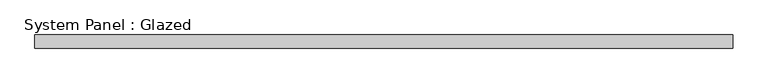
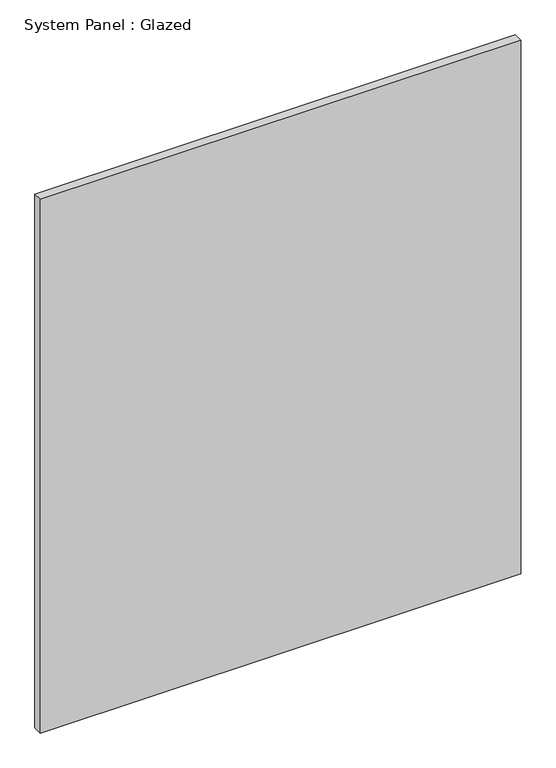
"""IFC4 building model written with IfcOpenShell, lengths in millimetres: plate geometry, System Panel : Glazed."""

from ifc_helpers import new_model, si_unit, origin, origin_with_axes, place, context, project, spatial, polyline, outline, extrude, source, transform, mapped, element, save


def system_panel_glazed_4af92da9(model_context):
    return source(origin(), model_context, "Body", "SweptSolid", [
        extrude(outline(polyline([(654.05, 19.05), (-654.05, 19.05), (-654.05, 44.45), (654.05, 44.45), (654.05, 19.05)])), origin_with_axes(), (0.0, 0.0, 1.0), 1535.7829369),
    ])


if __name__ == "__main__":
    model = new_model("IFC4")
    model_context = context("Model", 3, world=origin())
    ifc_project = project(units=[si_unit("LENGTHUNIT", "METRE", prefix="MILLI")], contexts=[model_context])
    site = spatial("IfcSite", under=ifc_project)
    building = spatial("IfcBuilding", under=site)
    placement = place(None, origin())
    system_panel_glazed_shape = system_panel_glazed_4af92da9(model_context)
    element("IfcPlate", 1, ObjectType="System Panel : Glazed", at=placement, inside=building, context=model_context, shape_type="MappedRepresentation", body=[
        mapped(system_panel_glazed_shape, transform((0.0, 0.0, 0.0), x_axis=(1.0, 0.0, 0.0), y_axis=(0.0, 1.0, 0.0), z_axis=(0.0, 0.0, 1.0))),
    ])
    save(model, "model.ifc")

# Revit data of these elements
# Type "System Panel : Glazed"
#   Construction Type Id = "GSP4R"
#   Analytic Construction = "1/8 in Pilkington single glazing"
#   Visual Light Transmittance = 0.9
#   Solar Heat Gain Coefficient = 0.86
#   Heat Transfer Coefficient (U) = 1.18115 BTU/(h·ft²·°F)
#   Define Thermal Properties by = 1
# Element 1 (IfcPlate, "System Panel : Glazed")
#   Materials on its faces: "Glass"
# Materials
#   "Glass": class "Glass", colour RGB 0 128 192, transparency 0.75, Description = "Soda Lime Glass", Cost = 0
